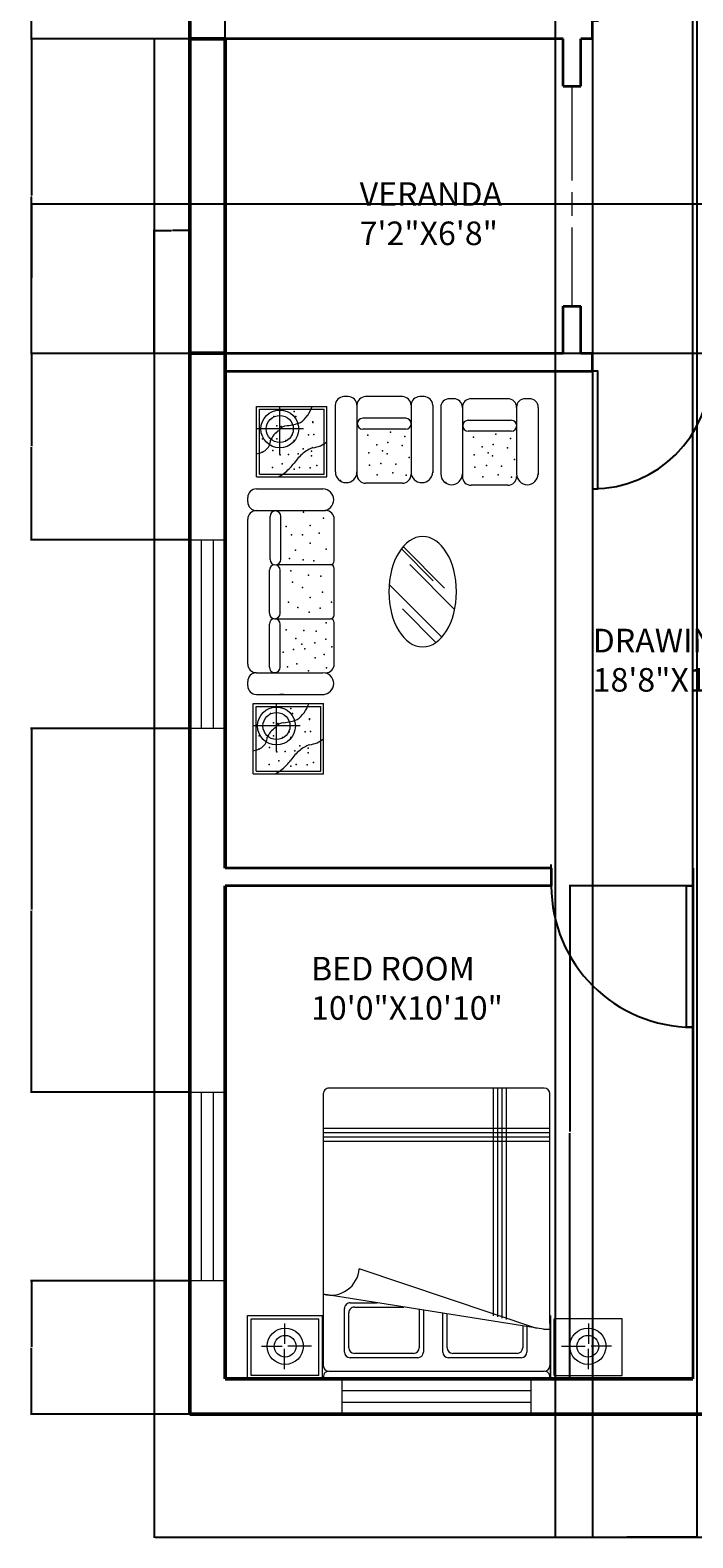
# Model space of a CAD drawing. Units: feet. Extents: x 2664 to 3060, y 1318 to 2005.
# Tile 1 of 5: x 2664 to 2832, y 1318 to 1702. Entities that reach past the tile are written whole.
import ezdxf

# ---------------------------------------------------------------- set-up
doc = ezdxf.new("R2010")
doc.units = ezdxf.units.FT
doc.linetypes.add('ACAD_ISO08W100', pattern=[36, 24, -3, 6, -3])
for name, color, linetype, lineweight in [('A-ANNO-DIMS', 2, 'Continuous', 18), ('A-AREA-IDEN', 109, 'Continuous', 18), ('A-WALL-EXTR', 130, 'Continuous', 50), ('DOOR', 249, 'Continuous', 25), ('FURNITURE', 240, 'Continuous', 13), ('STAIR', 182, 'Continuous', 25)]:
    doc.layers.add(name, color=color, linetype=linetype, lineweight=lineweight)
for name, color, linetype, lineweight, true_color in [('A-FLOR-GRIL', 222, 'ACAD_ISO08W100', 18, 0xd4008b), ('A-GLAZ', 222, 'Continuous', 18, 0xd4008b), ('A-WALL-INTR', 41, 'Continuous', 35, 0xf5dd7a)]:
    doc.layers.add(name, color=color, linetype=linetype, lineweight=lineweight, true_color=true_color)
doc.styles.get("Standard").update_dxf_attribs({"font": 'arial.ttf'})
doc.dimstyles.get("Standard").update_dxf_attribs({"dimtxt": 0.18, "dimasz": 0.18, "dimexe": 0.18, "dimexo": 0.0625, "dimgap": 0.09, "dimtad": 0, "dimtih": 1, "dimtoh": 1, "dimdec": 4, "dimzin": 0, "dimdsep": 46, "dimtxsty": 'Standard', "dimcen": 0.09, "dimadec": 0, "dimazin": 0, "dimtfac": 1, "dimtdec": 4, "dimtofl": 0, "dimtmove": 0, "dimatfit": 3, "dimfxl": 1, "dimtolj": 1, "dimtzin": 0, "dimarcsym": 0})

# ---------------------------------------------------------------- blocks, each defined once
blk = doc.blocks.new('*U5')
for p, q in [((-40, 0), (-40, 6)), ((0, 0), (0, 6))]:
    blk.add_line(p, q)
blk.add_lwpolyline([(0, 0), (0, -40), (-1.75, -40), (-1.75, 0)], close=True)
blk.add_arc((0, 0), 40, 180, 270)
blk = doc.blocks.new('*U2')
for p, q in [((0, 0), (0, -6)), ((40, 0), (40, -6))]:
    blk.add_line(p, q)
blk.add_lwpolyline([(0, 0), (0, 40), (1.75, 40), (1.75, 0)], close=True)
blk.add_arc((0, 0), 40, 0, 90)
blk = doc.blocks.new('*U6')
for p, q in [((0, 0), (0, 6)), ((40, 0), (40, 6))]:
    blk.add_line(p, q)
blk.add_lwpolyline([(0, 0), (0, -40), (1.75, -40), (1.75, 0)], close=True)
blk.add_arc((0, 0), 40, 270, 0)
blk = doc.blocks.new('TABLE-END')
for p, q in [((-8.83, -9), (-8.83, 8.9)), ((-8.83, 8.9), (9.06, 8.9)), ((-8.14, -8.31), (-8.14, 8.21)), ((-8.14, 8.21), (8.38, 8.21)), ((-2.94, -3.32), (-2.94, 9)), ((8.38, -8.31), (8.38, 8.21)), ((9.06, -9), (9.06, 8.9)), ((3.1, 3.21), (-8.97, 3.21)), ((-8.83, -9), (9.06, -9)), ((-8.14, -8.31), (8.38, -8.31))]:
    blk.add_line(p, q)
for radius in [4.81, 3.44]:
    blk.add_circle((-2.94, 3.21), radius)
for centre, radius, start, end in [((-3.5, 11.98), 9.32, 324.6463, 340.6785), ((-0.75, 0.94), 3.12, 96.1016, 144.1315), ((-2.19, 16.41), 12.41, 275.1129, 291.2782), ((-1.58, 10.62), 6.96, 304.0039, 324.6463), ((-8.44, 0.34), 3.14, 305.9664, 0.3439), ((0.7, -2.61), 6.69, 126.4548, 153.626), ((-9.98, 3.26), 6.46, 278.1279, 293.3746), ((-9.12, 1.28), 4.31, 293.3746, 305.9664), ((12.46, -14.07), 14.57, 130.5005, 143.836), ((8.07, -8.93), 7.82, 109.24, 130.5005), ((4.71, 5.19), 6.79, 276.623, 309.8575), ((-9.43, 1.93), 12.54, 309.4558, 323.836), ((-7.51, -0.4), 9.52, 297.4626, 309.4558)]:
    blk.add_arc(centre, radius, start, end)
for p in [(-4.49, 6.42), (-3.72, 3.98), (0.71, 7.64), (1.18, 6.4), (5.44, 5.05), (5.44, 4.89), (-7.32, 0.7), (-3.69, 0.7), (-2.55, 3.81), (-1.43, 0.31), (0.25, 1.69), (0.71, 0.31), (4.37, 1.69), (5.75, 1.84), (-7.41, -2.67), (-4.73, -2.3), (-2.81, -3.35), (-0.75, -3.26), (1.74, -3.15), (3, -1.82), (5.12, -2.41), (5.14, -3.65), (-4.79, -6.56), (-2.35, -5.64), (0.72, -7.03), (2.08, -6.56), (4.83, -6.71), (6.51, -6.1)]:
    blk.add_point(p)
blk = doc.blocks.new('SOFA-3-SEAT')
for p, q in [((-11.01, -3.3), (-11.01, -2.2)), ((-8.81, 0), (8.12, 0)), ((-8.81, -5.51), (-4.95, -5.51)), ((-5.34, -17.95), (-5.34, -6.98)), ((-4.95, -5.51), (8.81, -5.51)), ((-2.59, -17.95), (-2.59, -6.98)), ((-11.01, -44.59), (-11.01, -7.71)), ((11.01, -18.31), (11.01, -7.71)), ((-5.51, -31.66), (-5.51, -20.69)), ((-3.58, -19.27), (10.05, -19.27)), ((-2.75, -31.66), (-2.75, -20.69)), ((11.01, -32.07), (11.01, -20.23)), ((-5.51, -45.38), (-5.51, -34.41)), ((-4.13, -33.03), (10.05, -33.03)), ((-2.75, -45.38), (-2.75, -34.41)), ((11.01, -44.59), (11.01, -34.04)), ((-11.01, -50.1), (-11.01, -49)), ((-8.81, -46.8), (8.12, -46.8)), ((-8.81, -52.3), (8.4, -52.3)), ((-2.79, -52.3), (-2.81, -52.3)), ((-1.79, -52.3), (-2.79, -52.3))]:
    blk.add_line(p, q)
for centre, radius, start, end in [((-8.81, -2.2), 2.2, 90, 180), ((-8.81, -3.3), 2.2, 180, 270), ((8.12, -2.75), 2.75, 0, 90), ((8.12, -2.75), 2.75, 270, 0), ((-8.81, -7.71), 2.2, 90, 180), ((-3.96, -6.98), 1.38, 90, 180), ((-3.96, -6.98), 1.38, 0, 90), ((8.81, -7.71), 2.2, 0, 90), ((-3.96, -17.95), 1.38, 180, 270), ((-3.96, -17.95), 1.38, 270, 0), ((10.05, -18.31), 0.963, 270, 0), ((-4.13, -20.69), 1.38, 90, 180), ((-4.13, -20.69), 1.38, 0, 90), ((10.05, -20.23), 0.963, 0, 90), ((-4.13, -31.66), 1.38, 180, 270), ((-4.13, -34.41), 1.38, 90, 180), ((-4.13, -31.66), 1.38, 270, 0), ((-4.13, -34.41), 1.38, 0, 90), ((10.05, -32.07), 0.963, 270, 0), ((10.05, -34.04), 0.963, 0, 90), ((-8.81, -44.59), 2.2, 180, 270), ((-4.13, -45.38), 1.38, 180, 270), ((-4.13, -45.38), 1.38, 270, 0), ((8.81, -44.59), 2.2, 270, 0), ((-8.81, -49), 2.2, 90, 180), ((8.12, -49.55), 2.75, 0, 90), ((8.12, -49.55), 2.75, 270, 0), ((-8.81, -50.1), 2.2, 180, 270), ((-2.76, -44.04), 8.26, 268.9725, 269.066), ((-2.75, -42.86), 9.44, 269.1265, 269.4492), ((-2.75, -44.04), 8.26, 269.411, 269.6618), ((-2.78, -44.04), 8.26, 269.9826, 270)]:
    blk.add_arc(centre, radius, start, end)
for p in [(3.15, -5.94), (8.25, -7.42), (-1.22, -9.57), (4.85, -9.35), (7.19, -11.26), (0.16, -11.65), (2.9, -11.65), (4.85, -13.8), (-0.42, -17.7), (1.14, -15.55), (3.09, -18.09), (5.82, -18.28), (8.94, -15.36), (-0.03, -20.82), (4.46, -21.98), (7.58, -22.18), (0.36, -23.74), (2.9, -25.1), (7.97, -26.27), (-0.62, -28.81), (1.73, -30.17), (4.85, -27.64), (7.38, -30.37), (10.31, -28.81), (4.65, -31.34), (8.94, -34.07), (-1.2, -35.83), (1.22, -38.06), (3.29, -36.02), (6.41, -36.22), (8.84, -38.21), (-1.96, -41.54), (0.63, -40.87), (2.78, -39.55), (3.52, -40.73), (6.02, -39.14), (8.4, -42.13), (10.4, -40.21), (-0.85, -45.24), (1.44, -44.5), (6.18, -42.95), (8.99, -45.54), (4.48, -46.28)]:
    blk.add_point(p)
blk = doc.blocks.new('TABLE-COFFEE-OVAL')
for p, q in [((2.67, 2.77), (-5.41, 10.92)), ((5.56, 0.91), (-4.93, 11.5)), ((8.13, -4.53), (-3.25, 6.96)), ((4.85, -11.6), (-8.51, 1.88)), ((3.36, -12.93), (-5.15, -4.35))]:
    blk.add_line(p, q)
at = {"extrusion": (0, 0, -1)}
blk.add_ellipse((0, 0), major_axis=(0, 14.05), ratio=0.611621, dxfattribs=at)
blk = doc.blocks.new('CHAIR-ARM')
for p, q in [((-9.08, 0), (-10.19, 0)), ((4.68, 0), (-4.68, 0)), ((10.19, 0), (9.08, 0)), ((-12.39, -2.2), (-12.39, -19.13)), ((-6.88, -2.2), (-6.88, -6.06)), ((-6.88, -2.2), (-6.88, -6.12)), ((-6.88, -2.2), (-6.88, -19.82)), ((6.88, -2.2), (6.88, -19.13)), ((12.39, -2.2), (12.39, -19.41)), ((5.54, -5.51), (-5.43, -5.51)), ((5.54, -8.26), (-5.43, -8.26)), ((4.68, -8.26), (-4.68, -8.26)), ((4.68, -22.02), (-4.68, -22.02))]:
    blk.add_line(p, q)
for centre, radius, start, end in [((-10.19, -2.2), 2.2, 90, 180), ((-9.08, -2.2), 2.2, 0, 90), ((-4.68, -2.2), 2.2, 90, 180), ((4.68, -2.2), 2.2, 0, 90), ((9.08, -2.2), 2.2, 90, 180), ((10.19, -2.2), 2.2, 0, 90), ((-5.43, -6.88), 1.38, 90, 180), ((-5.43, -6.88), 1.38, 180, 270), ((5.54, -6.88), 1.38, 0, 90), ((5.54, -6.88), 1.38, 270, 0), ((-9.63, -19.13), 2.75, 180, 270), ((-9.63, -19.13), 2.75, 270, 0), ((9.63, -19.13), 2.75, 180, 270), ((9.63, -19.13), 2.75, 270, 0), ((-4.68, -19.82), 2.2, 180, 270), ((4.68, -19.82), 2.2, 270, 0)]:
    blk.add_arc(centre, radius, start, end)
for p in [(-4.09, -9.81), (1.63, -9.05), (5.33, -10.16), (-3.89, -14.3), (-1.86, -12.23), (-0.36, -13.79), (0.81, -14.53), (0.96, -11.64), (4.59, -12.46), (-3.7, -17.42), (-0.77, -17.03), (3.03, -17.19), (6.36, -15.49), (-11.11, -21.32), (-1.71, -19.86), (2.22, -19.41), (5.62, -20)]:
    blk.add_point(p)
blk = doc.blocks.new('BED-DOUBLE-WITH-NIGHTSTANDS')
for p, q in [((-29.54, 0), (-29.54, -16.21)), ((-30.37, -0.95), (-47.65, -0.95)), ((-47.65, -0.95), (-47.65, -15.35)), ((-39.11, -2.58), (-39.11, -7.74)), ((-30.37, -0.95), (-30.37, -15.35)), ((-29.47, -0.05), (-29.47, -16.25)), ((-29.26, -14.16), (-29.26, -3.5)), ((28.27, -0.11), (-29.17, -0.11)), ((26.92, -2.06), (-27.82, -2.06)), ((28.36, -72.65), (28.36, -3.5)), ((28.57, -0.05), (47.65, -0.05)), ((28.57, -0.05), (28.57, -16.25)), ((29.47, -0.95), (46.75, -0.95)), ((29.47, -0.95), (29.47, -15.35)), ((38.21, -2.58), (38.21, -7.74)), ((46.75, -0.95), (46.75, -15.35)), ((47.65, -0.05), (47.65, -16.25)), ((-23.45, -13.32), (-23.45, -6.94)), ((-22.01, -5.5), (-3.48, -5.5)), ((-20.93, -6.58), (-4.56, -6.58)), ((-2.04, -6.94), (-2.04, -16.8)), ((2.88, -17.58), (2.88, -6.94)), ((4.33, -5.5), (21.52, -5.5)), ((5.41, -6.58), (20.44, -6.58)), ((22.96, -6.94), (22.96, -18.02)), ((-44.95, -8.46), (-39.75, -8.46)), ((-39.11, -14.22), (-39.11, -9.06)), ((-32.27, -8.46), (-38.27, -8.46)), ((-22.37, -13.47), (-22.37, -8.02)), ((-3.12, -8.02), (-3.12, -16.63)), ((3.96, -17.76), (3.96, -8.02)), ((21.88, -8.02), (21.88, -16.94)), ((31.37, -8.46), (37.37, -8.46)), ((38.21, -14.22), (38.21, -9.06)), ((44.05, -8.46), (38.85, -8.46)), ((-27.62, -12.73), (-29.26, -12.73)), ((-29.26, -14.16), (-29.26, -72.65)), ((-27.62, -12.73), (28.36, -21.64)), ((-26, -12.96), (19.2, -28.15)), ((-18.14, -74.09), (-18.14, -15.24)), ((-47.65, -15.35), (-30.37, -15.35)), ((-17.06, -74.09), (-17.06, -15.55)), ((-15.97, -74.09), (-15.97, -15.86)), ((-14.89, -74.09), (-14.89, -16.18)), ((20.44, -18.38), (7.87, -18.38)), ((47.65, -16.25), (28.57, -16.25)), ((46.75, -15.35), (29.47, -15.35)), ((21.52, -19.46), (14.66, -19.46)), ((28.36, -60.64), (-29.26, -60.64)), ((28.36, -61.72), (-29.26, -61.72)), ((28.36, -62.8), (-29.26, -62.8)), ((28.36, -63.88), (-29.26, -63.88)), ((-27.82, -74.09), (26.92, -74.09))]:
    blk.add_line(p, q)
for centre, radius in [((-38.95, -8.4), 4.61), ((38.05, -8.4), 4.61), ((-38.95, -8.4), 2.77), ((38.05, -8.4), 2.77)]:
    blk.add_circle(centre, radius)
for centre, radius, start, end in [((-27.82, -0.62), 1.44, 159.2884, 270), ((-27.82, -3.5), 1.44, 90, 180), ((26.92, -0.62), 1.44, 270, 20.7116), ((26.92, -3.5), 1.44, 0, 90), ((-22.01, -6.94), 1.44, 90, 180), ((-20.93, -8.02), 1.44, 90, 180), ((-4.56, -8.02), 1.44, 0, 90), ((-3.48, -6.94), 1.44, 0, 90), ((4.33, -6.94), 1.44, 90, 180), ((5.41, -8.02), 1.44, 90, 180), ((20.44, -8.02), 1.44, 0, 90), ((21.52, -6.94), 1.44, 0, 90), ((20.44, -16.94), 1.44, 270, 0), ((21.52, -18.02), 1.44, 270, 0), ((26.5, -28.71), 7.32, 75.237, 175.5647), ((-27.82, -72.65), 1.44, 180, 270), ((26.92, -72.65), 1.44, 270, 0)]:
    blk.add_arc(centre, radius, start, end)
blk = doc.blocks.new('WINDOW-4FT')
for p, q in [((-24, 4.5), (24, 4.5)), ((-24, -4.5), (-24, 4.5)), ((24, 4.5), (24, -4.5)), ((-24, 1.5), (24, 1.5)), ((24, -1.5), (-24, -1.5)), ((24, -4.5), (-24, -4.5))]:
    blk.add_line(p, q)
blk = doc.blocks.new('*D32')
at = {"layer": 'A-ANNO-DIMS', "color": 0, "lineweight": -2, "transparency": 16777216}
for p, q in [((2695.28, 1619.51), (2695.28, 1318.11)), ((3028.28, 1349.51), (3028.28, 1318.11)), ((2695.46, 1318.29), (2861.49, 1318.29)), ((3028.1, 1318.29), (2862.07, 1318.29))]:
    blk.add_line(p, q, dxfattribs=at)
at = {"layer": 'A-ANNO-DIMS', "color": 0, "transparency": 16777216}
for points in [[(2695.46, 1318.32), (2695.46, 1318.26), (2695.28, 1318.29)], [(3028.1, 1318.32), (3028.1, 1318.26), (3028.28, 1318.29)]]:
    blk.add_solid(points, dxfattribs=at)
at = {"layer": 'Defpoints', "color": 0, "transparency": 16777216}
for p in [(2695.28, 1619.57), (3028.28, 1349.57), (3028.28, 1318.29)]:
    blk.add_point(p, dxfattribs=at)
at = {"layer": 'A-ANNO-DIMS', "color": 0, "transparency": 16777216, "insert": (2861.78, 1318.29), "char_height": 0.18, "attachment_point": 5}
blk.add_mtext('\\A1;333', dxfattribs=at)
blk = doc.blocks.new('*D34')
at = {"layer": 'A-ANNO-DIMS', "color": 0, "lineweight": -2, "transparency": 16777216}
for p, q in [((2695.28, 1619.63), (2695.28, 1651.03)), ((2695.46, 1650.85), (2699.63, 1650.85)), ((2704.1, 1650.85), (2699.93, 1650.85)), ((2704.28, 1619.63), (2704.28, 1651.03))]:
    blk.add_line(p, q, dxfattribs=at)
at = {"layer": 'A-ANNO-DIMS', "color": 0, "transparency": 16777216}
for points in [[(2695.46, 1650.88), (2695.46, 1650.82), (2695.28, 1650.85)], [(2704.1, 1650.88), (2704.1, 1650.82), (2704.28, 1650.85)]]:
    blk.add_solid(points, dxfattribs=at)
at = {"layer": 'Defpoints', "color": 0, "transparency": 16777216}
for p in [(2704.28, 1650.85), (2695.28, 1619.57), (2704.28, 1619.57)]:
    blk.add_point(p, dxfattribs=at)
at = {"layer": 'A-ANNO-DIMS', "color": 0, "transparency": 16777216, "insert": (2699.78, 1650.85), "char_height": 0.18, "attachment_point": 5}
blk.add_mtext('\\A1;9', dxfattribs=at)
blk = doc.blocks.new('*D42')
at = {"layer": 'A-ANNO-DIMS', "color": 0, "lineweight": -2, "transparency": 16777216}
for p, q in [((2704.22, 1755.77), (2663.82, 1755.77)), ((2664, 1755.59), (2664, 1727.85)), ((2664, 1699.75), (2664, 1727.49)), ((2704.22, 1699.57), (2663.82, 1699.57))]:
    blk.add_line(p, q, dxfattribs=at)
at = {"layer": 'A-ANNO-DIMS', "color": 0, "transparency": 16777216}
for points in [[(2663.97, 1755.59), (2664.03, 1755.59), (2664, 1755.77)], [(2663.97, 1699.75), (2664.03, 1699.75), (2664, 1699.57)]]:
    blk.add_solid(points, dxfattribs=at)
at = {"layer": 'Defpoints', "color": 0, "transparency": 16777216}
for p in [(2704.28, 1755.77), (2664, 1699.57), (2704.28, 1699.57)]:
    blk.add_point(p, dxfattribs=at)
at = {"layer": 'A-ANNO-DIMS', "color": 0, "transparency": 16777216, "insert": (2664, 1727.67), "char_height": 0.18, "attachment_point": 5}
blk.add_mtext('\\A1;56.2', dxfattribs=at)
blk = doc.blocks.new('*D43')
at = {"layer": 'A-ANNO-DIMS', "color": 0, "lineweight": -2, "transparency": 16777216}
for p, q in [((2695.22, 1699.57), (2663.82, 1699.57)), ((2664, 1699.39), (2664, 1659.75)), ((2664, 1619.75), (2664, 1659.39)), ((2695.22, 1619.57), (2663.82, 1619.57))]:
    blk.add_line(p, q, dxfattribs=at)
at = {"layer": 'A-ANNO-DIMS', "color": 0, "transparency": 16777216}
for points in [[(2663.97, 1699.39), (2664.03, 1699.39), (2664, 1699.57)], [(2663.97, 1619.75), (2664.03, 1619.75), (2664, 1619.57)]]:
    blk.add_solid(points, dxfattribs=at)
at = {"layer": 'Defpoints', "color": 0, "transparency": 16777216}
for p in [(2695.28, 1699.57), (2664, 1619.57), (2695.28, 1619.57)]:
    blk.add_point(p, dxfattribs=at)
at = {"layer": 'A-ANNO-DIMS', "color": 0, "transparency": 16777216, "insert": (2664, 1659.57), "char_height": 0.18, "attachment_point": 5}
blk.add_mtext('\\A1;80', dxfattribs=at)
blk = doc.blocks.new('*D44')
at = {"layer": 'A-ANNO-DIMS', "color": 0, "lineweight": -2, "transparency": 16777216}
for p, q in [((2704.22, 1619.57), (2663.82, 1619.57)), ((2664, 1619.39), (2664, 1596.02)), ((2664, 1572.29), (2664, 1595.66)), ((2704.22, 1572.11), (2663.82, 1572.11))]:
    blk.add_line(p, q, dxfattribs=at)
at = {"layer": 'A-ANNO-DIMS', "color": 0, "transparency": 16777216}
for points in [[(2663.97, 1619.39), (2664.03, 1619.39), (2664, 1619.57)], [(2663.97, 1572.29), (2664.03, 1572.29), (2664, 1572.11)]]:
    blk.add_solid(points, dxfattribs=at)
at = {"layer": 'Defpoints', "color": 0, "transparency": 16777216}
for p in [(2704.28, 1619.57), (2664, 1572.11), (2704.28, 1572.11)]:
    blk.add_point(p, dxfattribs=at)
at = {"layer": 'A-ANNO-DIMS', "color": 0, "transparency": 16777216, "insert": (2664, 1595.84), "char_height": 0.18, "attachment_point": 5}
blk.add_mtext('\\A1;47.46', dxfattribs=at)
blk = doc.blocks.new('*D45')
at = {"layer": 'A-ANNO-DIMS', "color": 0, "lineweight": -2, "transparency": 16777216}
for p, q in [((2704.22, 1524.11), (2663.82, 1524.11)), ((2664, 1523.93), (2664, 1478.01)), ((2664, 1431.73), (2664, 1477.65)), ((2704.22, 1431.55), (2663.82, 1431.55))]:
    blk.add_line(p, q, dxfattribs=at)
at = {"layer": 'A-ANNO-DIMS', "color": 0, "transparency": 16777216}
for points in [[(2663.97, 1523.93), (2664.03, 1523.93), (2664, 1524.11)], [(2663.97, 1431.73), (2664.03, 1431.73), (2664, 1431.55)]]:
    blk.add_solid(points, dxfattribs=at)
at = {"layer": 'Defpoints', "color": 0, "transparency": 16777216}
for p in [(2704.28, 1524.11), (2664, 1431.55), (2704.28, 1431.55)]:
    blk.add_point(p, dxfattribs=at)
at = {"layer": 'A-ANNO-DIMS', "color": 0, "transparency": 16777216, "insert": (2664, 1477.83), "char_height": 0.18, "attachment_point": 5}
blk.add_mtext('\\A1;92.56', dxfattribs=at)
blk = doc.blocks.new('*D46')
at = {"layer": 'A-ANNO-DIMS', "color": 0, "lineweight": -2, "transparency": 16777216}
for p, q in [((2704.22, 1383.55), (2663.82, 1383.55)), ((2664, 1383.37), (2664, 1366.74)), ((2664, 1349.75), (2664, 1366.38)), ((2704.22, 1349.57), (2663.82, 1349.57))]:
    blk.add_line(p, q, dxfattribs=at)
at = {"layer": 'A-ANNO-DIMS', "color": 0, "transparency": 16777216}
for points in [[(2663.97, 1383.37), (2664.03, 1383.37), (2664, 1383.55)], [(2663.97, 1349.75), (2664.03, 1349.75), (2664, 1349.57)]]:
    blk.add_solid(points, dxfattribs=at)
at = {"layer": 'Defpoints', "color": 0, "transparency": 16777216}
for p in [(2704.28, 1383.55), (2664, 1349.57), (2704.28, 1349.57)]:
    blk.add_point(p, dxfattribs=at)
at = {"layer": 'A-ANNO-DIMS', "color": 0, "transparency": 16777216, "insert": (2664, 1366.56), "char_height": 0.18, "attachment_point": 5}
blk.add_mtext('\\A1;33.98', dxfattribs=at)
blk = doc.blocks.new('*D50')
at = {"layer": 'A-ANNO-DIMS', "color": 0, "lineweight": -2, "transparency": 16777216}
for p, q in [((2879.47, 1657.57), (2663.82, 1657.57)), ((2664, 1657.39), (2664, 1638.75)), ((2664, 1619.75), (2664, 1638.39)), ((2879.47, 1619.57), (2663.82, 1619.57))]:
    blk.add_line(p, q, dxfattribs=at)
at = {"layer": 'A-ANNO-DIMS', "color": 0, "transparency": 16777216}
for points in [[(2663.97, 1657.39), (2664.03, 1657.39), (2664, 1657.57)], [(2663.97, 1619.75), (2664.03, 1619.75), (2664, 1619.57)]]:
    blk.add_solid(points, dxfattribs=at)
at = {"layer": 'Defpoints', "color": 0, "transparency": 16777216}
for p in [(2664, 1657.57), (2879.53, 1657.57), (2879.53, 1619.57)]:
    blk.add_point(p, dxfattribs=at)
at = {"layer": 'A-ANNO-DIMS', "color": 0, "transparency": 16777216, "insert": (2664, 1638.57), "char_height": 0.18, "attachment_point": 5}
blk.add_mtext('\\A1;38', dxfattribs=at)
blk = doc.blocks.new('*D51')
at = {"layer": 'A-ANNO-DIMS', "color": 0, "lineweight": -2, "transparency": 16777216}
for p, q in [((2806.78, 1699.51), (2806.78, 1318.11)), ((2866.78, 1699.51), (2866.78, 1318.11)), ((2806.96, 1318.29), (2836.56, 1318.29)), ((2866.6, 1318.29), (2837, 1318.29))]:
    blk.add_line(p, q, dxfattribs=at)
at = {"layer": 'A-ANNO-DIMS', "color": 0, "transparency": 16777216}
for points in [[(2806.96, 1318.32), (2806.96, 1318.26), (2806.78, 1318.29)], [(2866.6, 1318.32), (2866.6, 1318.26), (2866.78, 1318.29)]]:
    blk.add_solid(points, dxfattribs=at)
at = {"layer": 'Defpoints', "color": 0, "transparency": 16777216}
for p in [(2806.78, 1699.57), (2866.78, 1699.57), (2866.78, 1318.29)]:
    blk.add_point(p, dxfattribs=at)
at = {"layer": 'A-ANNO-DIMS', "color": 0, "transparency": 16777216, "insert": (2836.78, 1318.29), "char_height": 0.18, "attachment_point": 5}
blk.add_mtext('\\A1;60', dxfattribs=at)
blk = doc.blocks.new('*D53')
at = {"layer": 'A-ANNO-DIMS', "color": 0, "lineweight": -2, "transparency": 16777216}
for p, q in [((2797.28, 1830.01), (2797.28, 1318.11)), ((2833.28, 1830.01), (2833.28, 1318.11)), ((2797.46, 1318.29), (2815.06, 1318.29)), ((2833.1, 1318.29), (2815.5, 1318.29))]:
    blk.add_line(p, q, dxfattribs=at)
at = {"layer": 'A-ANNO-DIMS', "color": 0, "transparency": 16777216}
for points in [[(2797.46, 1318.32), (2797.46, 1318.26), (2797.28, 1318.29)], [(2833.1, 1318.32), (2833.1, 1318.26), (2833.28, 1318.29)]]:
    blk.add_solid(points, dxfattribs=at)
at = {"layer": 'Defpoints', "color": 0, "transparency": 16777216}
for p in [(2797.28, 1830.07), (2833.28, 1830.07), (2833.28, 1318.29)]:
    blk.add_point(p, dxfattribs=at)
at = {"layer": 'A-ANNO-DIMS', "color": 0, "transparency": 16777216, "insert": (2815.28, 1318.29), "char_height": 0.18, "attachment_point": 5}
blk.add_mtext('\\A1;36', dxfattribs=at)
blk = doc.blocks.new('*D59')
at = {"layer": 'A-ANNO-DIMS', "color": 0, "lineweight": -2, "transparency": 16777216}
for p, q in [((2713.28, 1488.63), (2713.28, 2005.03)), ((2713.46, 2004.85), (2772.5, 2004.85)), ((2832.1, 2004.85), (2773.06, 2004.85)), ((2832.28, 1489.53), (2832.28, 2005.03))]:
    blk.add_line(p, q, dxfattribs=at)
at = {"layer": 'A-ANNO-DIMS', "color": 0, "transparency": 16777216}
for points in [[(2713.46, 2004.88), (2713.46, 2004.82), (2713.28, 2004.85)], [(2832.1, 2004.88), (2832.1, 2004.82), (2832.28, 2004.85)]]:
    blk.add_solid(points, dxfattribs=at)
at = {"layer": 'Defpoints', "color": 0, "transparency": 16777216}
for p in [(2832.28, 2004.85), (2832.28, 1489.47), (2713.28, 1488.57)]:
    blk.add_point(p, dxfattribs=at)
at = {"layer": 'A-ANNO-DIMS', "color": 0, "transparency": 16777216, "insert": (2772.78, 2004.85), "char_height": 0.18, "attachment_point": 5}
blk.add_mtext('\\A1;119', dxfattribs=at)
blk = doc.blocks.new('*D60')
at = {"layer": 'A-ANNO-DIMS', "color": 0, "lineweight": -2, "transparency": 16777216}
for p, q in [((2832.22, 1484.07), (2800.82, 1484.07)), ((2801, 1483.89), (2801, 1421.5)), ((2801, 1358.75), (2801, 1421.14)), ((2832.22, 1358.57), (2800.82, 1358.57))]:
    blk.add_line(p, q, dxfattribs=at)
at = {"layer": 'A-ANNO-DIMS', "color": 0, "transparency": 16777216}
for points in [[(2800.97, 1483.89), (2801.03, 1483.89), (2801, 1484.07)], [(2800.97, 1358.75), (2801.03, 1358.75), (2801, 1358.57)]]:
    blk.add_solid(points, dxfattribs=at)
at = {"layer": 'Defpoints', "color": 0, "transparency": 16777216}
for p in [(2801, 1484.07), (2832.28, 1484.07), (2832.28, 1358.57)]:
    blk.add_point(p, dxfattribs=at)
at = {"layer": 'A-ANNO-DIMS', "color": 0, "transparency": 16777216, "insert": (2801, 1421.32), "char_height": 0.18, "attachment_point": 5}
blk.add_mtext('\\A1;125.5', dxfattribs=at)

msp = doc.modelspace()

# ---------------------------------------------------------------- linework, layer by layer
at = {"layer": 'A-FLOR-GRIL'}
msp.add_line((2801.53, 1687.571), (2801.53, 1631.571), dxfattribs=at)
at = {"layer": 'A-WALL-EXTR'}
for p, q in [((2704.28, 1349.571), (2704.28, 1973.571)), ((2713.28, 1699.571), (2704.28, 1699.571)), ((2713.28, 1488.571), (2713.28, 1699.571)), ((2704.28, 1619.571), (2713.28, 1619.571)), ((2713.28, 1358.571), (2713.28, 1484.071)), ((2832.28, 1358.571), (2713.28, 1358.571)), ((3028.28, 1349.571), (2704.28, 1349.571))]:
    msp.add_line(p, q, dxfattribs=at)
at = {"layer": 'A-WALL-INTR'}
for p, q in [((2806.78, 1699.571), (2806.78, 1704.071)), ((2799.28, 1699.571), (2713.28, 1699.571)), ((2799.28, 1687.571), (2799.28, 1699.571)), ((2806.78, 1699.571), (2803.78, 1699.571)), ((2803.78, 1687.571), (2803.78, 1699.571)), ((2799.28, 1687.571), (2803.78, 1687.571)), ((2799.28, 1619.571), (2799.28, 1631.571)), ((2799.28, 1631.571), (2803.78, 1631.571)), ((2803.78, 1619.571), (2803.78, 1631.571)), ((2713.28, 1619.571), (2799.28, 1619.571)), ((2713.28, 1619.571), (2799.28, 1619.571)), ((2803.78, 1619.571), (2806.78, 1619.571)), ((2803.78, 1619.571), (2806.78, 1619.571)), ((2806.78, 1615.071), (2806.78, 1619.571)), ((2713.28, 1615.071), (2799.28, 1615.071)), ((2799.28, 1615.071), (2803.78, 1615.071)), ((2803.78, 1615.071), (2806.78, 1615.071)), ((2796.28, 1488.571), (2713.28, 1488.571)), ((2796.28, 1488.571), (2796.28, 1484.071)), ((2832.28, 1488.571), (2832.28, 1358.571)), ((2796.28, 1484.071), (2713.28, 1484.071))]:
    msp.add_line(p, q, dxfattribs=at)
at = {"layer": 'STAIR'}
for p, q in [((2704.28, 1699.571), (2695.28, 1699.571)), ((2695.28, 1699.571), (2695.28, 1619.571)), ((2695.28, 1619.571), (2704.28, 1619.571))]:
    msp.add_line(p, q, dxfattribs=at)

# ---------------------------------------------------------------- block references
at = {"layer": 'A-GLAZ'}
for p, rotation in [((2708.78, 1548.11), 89.99999999999967), ((2708.78, 1407.55), 89.99999999999957), ((2767.081, 1354.071), 180)]:
    msp.add_blockref('WINDOW-4FT', p, dxfattribs=dict(at, rotation=rotation))
at = {"layer": 'DOOR'}
for name, p, xscale, yscale, zscale in [('*U2', (2806.78, 1704.071), 0.7500000000000038, 0.7500000000000038, 0.7500000000000038), ('*U6', (2806.78, 1615.071), 0.7500000000000038, 0.7500000000000038, 0.7500000000000038), ('*U5', (2832.28, 1484.071), 0.899999999999959, 0.899999999999959, 0.899999999999959)]:
    msp.add_blockref(name, p, dxfattribs=dict(at, xscale=xscale, yscale=yscale, zscale=zscale))
at = {"layer": 'FURNITURE'}
for name, p in [('CHAIR-ARM', (2753.715, 1608.544)), ('CHAIR-ARM', (2780.545, 1608.021)), ('TABLE-END', (2730.139, 1597.115)), ('SOFA-3-SEAT', (2730.053, 1585.066)), ('TABLE-COFFEE-OVAL', (2763.547, 1558.898)), ('TABLE-END', (2729.293, 1521.517))]:
    msp.add_blockref(name, p, dxfattribs=at)
at = {"layer": 'FURNITURE', "rotation": 180}
msp.add_blockref('BED-DOUBLE-WITH-NIGHTSTANDS', (2766.631, 1358.464), dxfattribs=at)

# ---------------------------------------------------------------- texts
at = {"layer": 'A-AREA-IDEN', "char_height": 6, "attachment_point": 1}
for s, width, insert in [('VERANDA\\P7\'2"X6\'8"', 22.955, (2747.52, 1663.117)), ('DRAWING \\P18\'8"X10\'6"', 22.955, (2806.796, 1549.47)), ('BED ROOM \\P10\'0"X10\'10"', 51.31518, (2735.146, 1465.969))]:
    msp.add_mtext_dynamic_manual_height_columns(s, width=width, gutter_width=12.5, heights=[0], dxfattribs=dict(at, insert=insert))

# ---------------------------------------------------------------- dimensions: what is measured, and where the dimension line sits
at = {"layer": 'A-ANNO-DIMS'}
for base, p1, p2, picture, middle in [((2832.28, 2004.851), (2713.28, 1488.571), (2832.28, 1489.471), '*D59', (2772.78, 2004.851)), ((2833.28, 1318.291), (2797.28, 1830.071), (2833.28, 1830.071), '*D53', (2815.28, 1318.291)), ((2866.78, 1318.291), (2806.78, 1699.571), (2866.78, 1699.571), '*D51', (2836.78, 1318.291)), ((2704.28, 1650.851), (2695.28, 1619.571), (2704.28, 1619.571), '*D34', (2699.78, 1650.851)), ((3028.28, 1318.291), (2695.28, 1619.571), (3028.28, 1349.571), '*D32', (2861.78, 1318.291))]:
    dim = msp.add_linear_dim(base=base, p1=p1, p2=p2, dimstyle='Standard', override={"dimdec": 0, "dimlfac": 1, "dimrnd": 0, "dimzin": 0, "dimdsep": 46, "dimlunit": 2}, dxfattribs=at)
    dim.commit()
    dim.dimension.update_dxf_attribs({"geometry": picture, "text_midpoint": middle})
for base, p1, p2, override, picture, middle in [((2664, 1699.571), (2704.28, 1755.772), (2704.28, 1699.571), {"dimdec": 1, "dimlfac": 1, "dimrnd": 0, "dimzin": 0, "dimdsep": 46, "dimlunit": 2}, '*D42', (2664, 1727.671)), ((2664, 1619.571), (2695.28, 1699.571), (2695.28, 1619.571), {"dimdec": 0, "dimlfac": 1, "dimrnd": 0, "dimzin": 0, "dimdsep": 46, "dimlunit": 2}, '*D43', (2664, 1659.571)), ((2664, 1657.571), (2879.53, 1619.571), (2879.53, 1657.571), {"dimdec": 0, "dimlfac": 1, "dimrnd": 0, "dimzin": 0, "dimdsep": 46, "dimlunit": 2}, '*D50', (2664, 1638.571)), ((2664, 1572.11), (2704.28, 1619.571), (2704.28, 1572.11), {"dimdec": 2, "dimlfac": 1, "dimrnd": 0, "dimzin": 0, "dimdsep": 46, "dimlunit": 2}, '*D44', (2664, 1595.84)), ((2664, 1431.55), (2704.28, 1524.11), (2704.28, 1431.55), {"dimdec": 2, "dimlfac": 1, "dimrnd": 0, "dimzin": 0, "dimdsep": 46, "dimlunit": 2}, '*D45', (2664, 1477.83)), ((2801, 1484.071), (2832.28, 1358.571), (2832.28, 1484.071), {"dimdec": 1, "dimlfac": 1, "dimrnd": 0, "dimzin": 0, "dimdsep": 46, "dimlunit": 2}, '*D60', (2801, 1421.321)), ((2664, 1349.571), (2704.28, 1383.55), (2704.28, 1349.571), {"dimdec": 2, "dimlfac": 1, "dimrnd": 0, "dimzin": 0, "dimdsep": 46, "dimlunit": 2}, '*D46', (2664, 1366.56))]:
    dim = msp.add_linear_dim(base=base, p1=p1, p2=p2, angle=90, dimstyle='Standard', override=override, dxfattribs=at)
    dim.commit()
    dim.dimension.update_dxf_attribs({"geometry": picture, "text_midpoint": middle})

doc.saveas('drawing.dxf')
